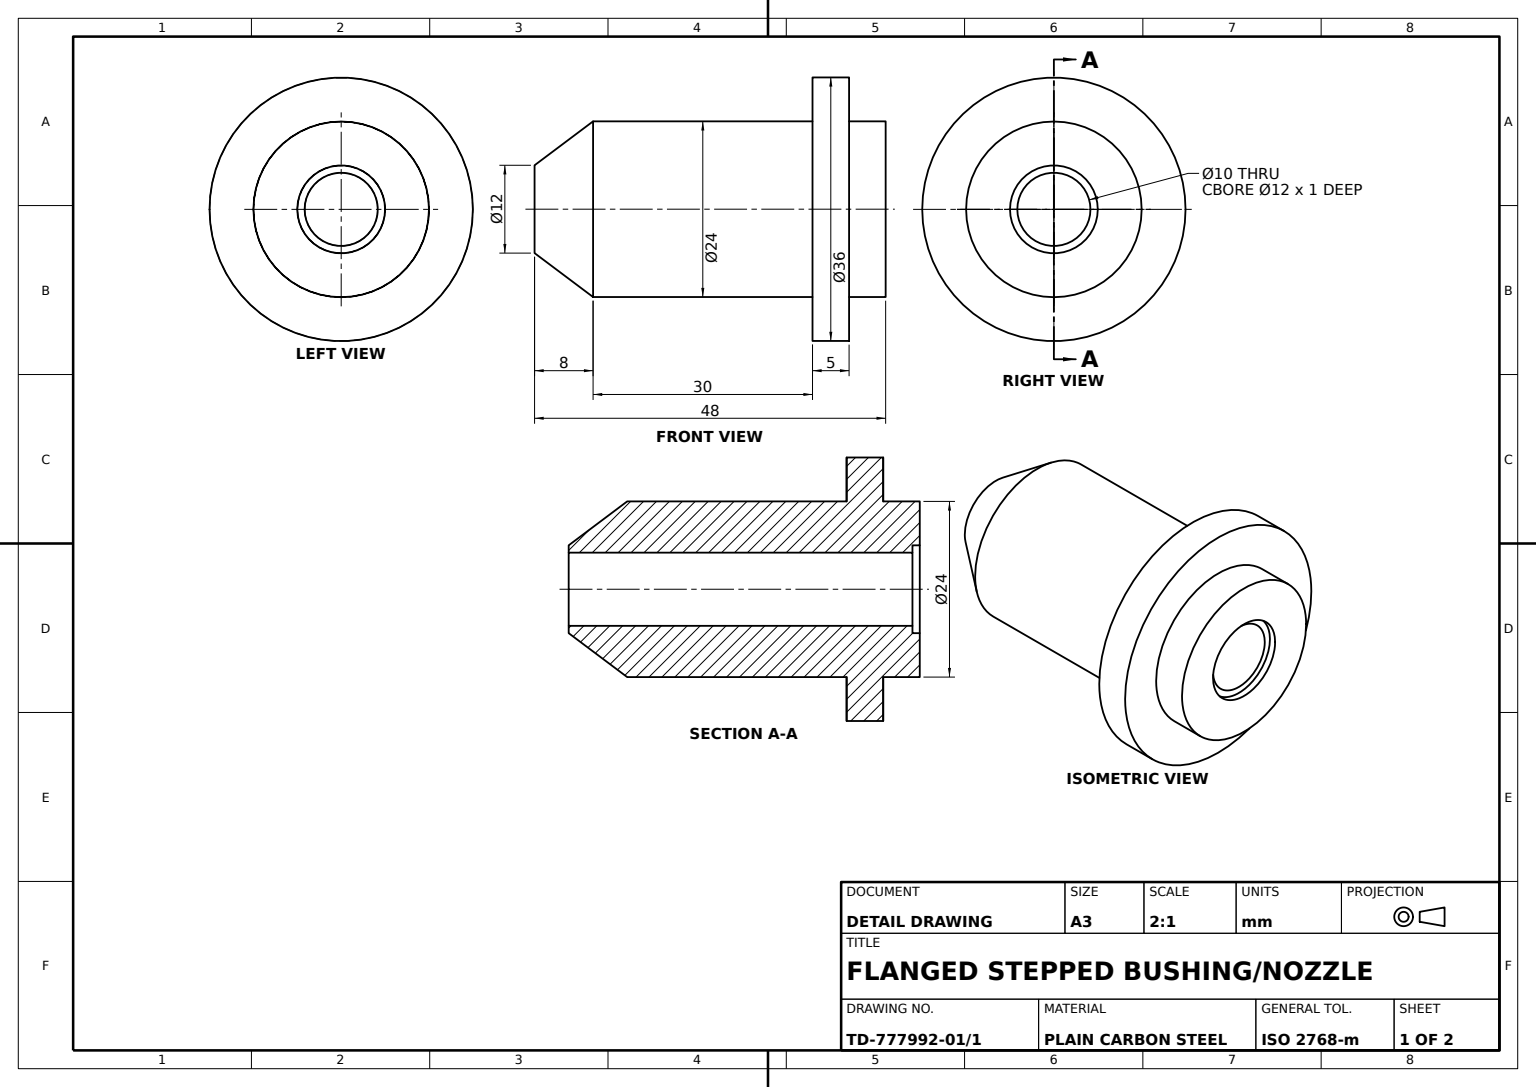
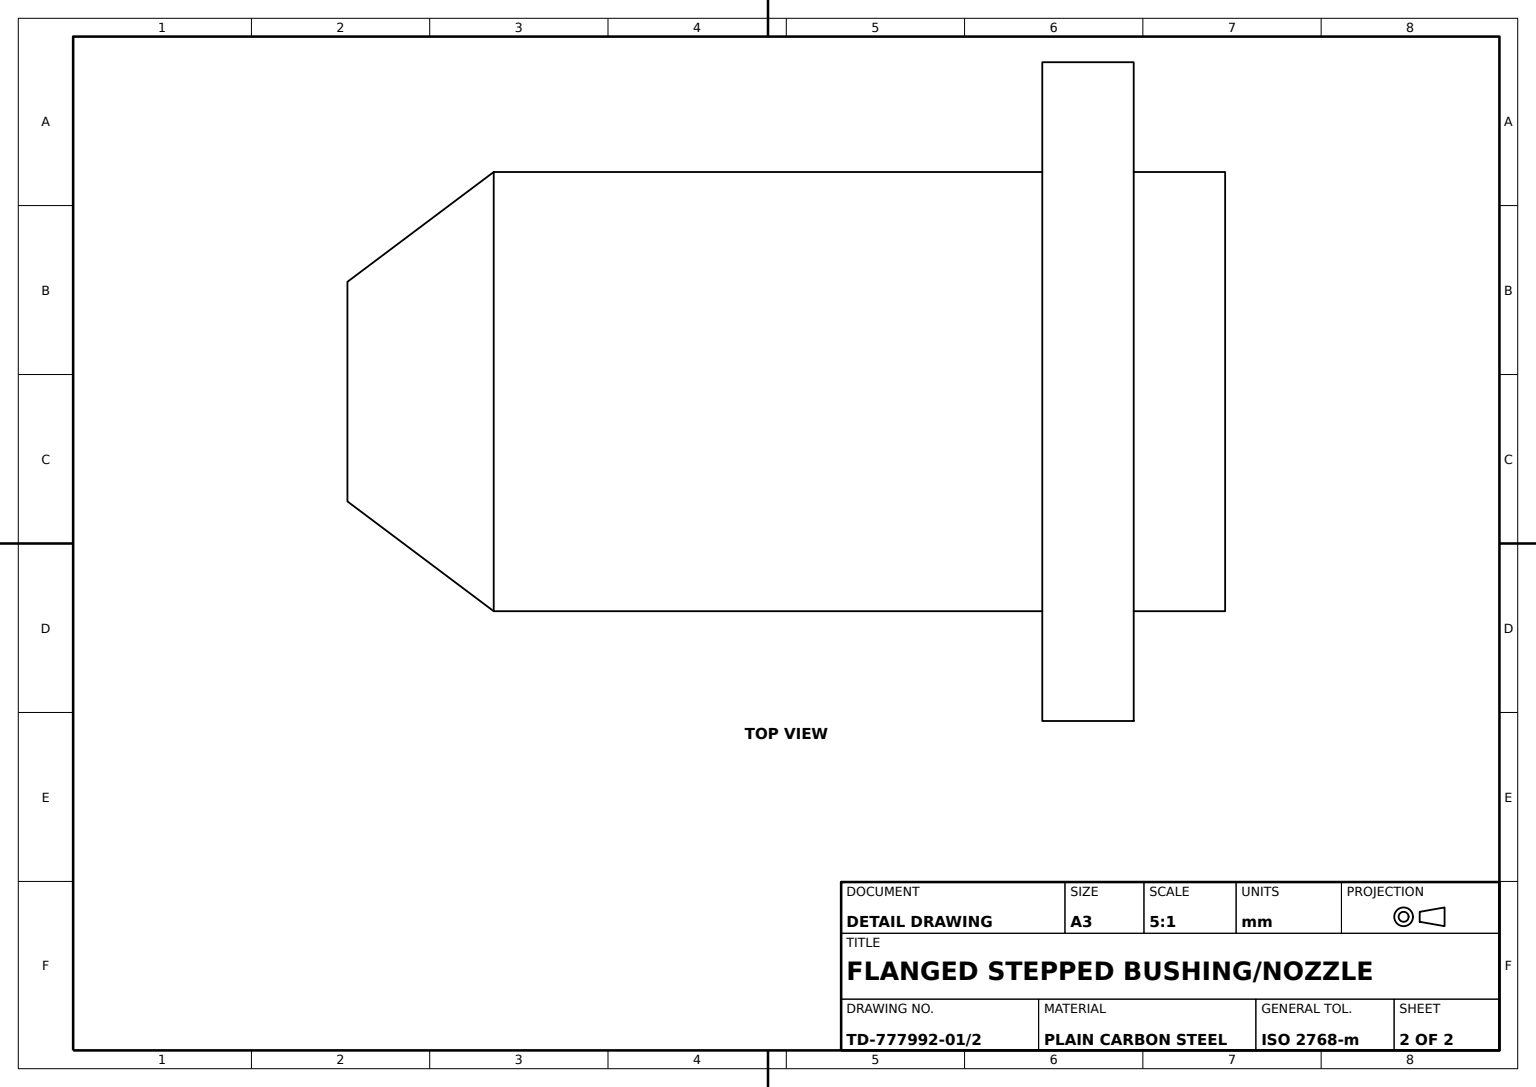
from build123d import *

# Parameters (mm, degrees)
COUNTERBORE_SKETCH_12_R = 6
COUNTERBORE_12X1_DEPTH  = 1
BORE_SKETCH_10_R        = 5
BORE_10X47_DEPTH        = 47


with BuildPart() as part:
    # Nozzle Profile Sketch → Nozzle Body Revolve (revolve)
    with BuildSketch(Plane.XY, mode=Mode.PRIVATE) as nozzle_body_revolve_sk:
        Polygon((0, 0), (0, 48), (-12, 48), (-12, 43), (-18, 43), (-18, 38), (-12, 38), (-12, 8), (-6, 0), align=None)
    revolve(nozzle_body_revolve_sk.sketch.rotate(Axis((0, 0, 0), (0, 1, 0)), 270), axis=Axis((0, 0, 0), (0, 1, 0)))

    # Counterbore Sketch Ø12 → Counterbore Ø12x1 (cut)
    with BuildSketch(Plane(origin=(0, 48, 0), x_dir=(1, 0, 0), z_dir=(0, 1, 0))):
        with Locations(Location((0, 0, 0), (0, 0, 270))):
            Circle(COUNTERBORE_SKETCH_12_R)
    extrude(amount=-COUNTERBORE_12X1_DEPTH, mode=Mode.SUBTRACT)

    # Bore Sketch Ø10 → Bore Ø10x47 (cut)
    with BuildSketch(Plane(origin=(0, 47, 0), x_dir=(1, 0, 0), z_dir=(0, 1, 0))):
        with Locations(Location((0, 0, 0), (0, 0, 270))):
            Circle(BORE_SKETCH_10_R)
    extrude(amount=-BORE_10X47_DEPTH, mode=Mode.SUBTRACT)


solid = part.part
